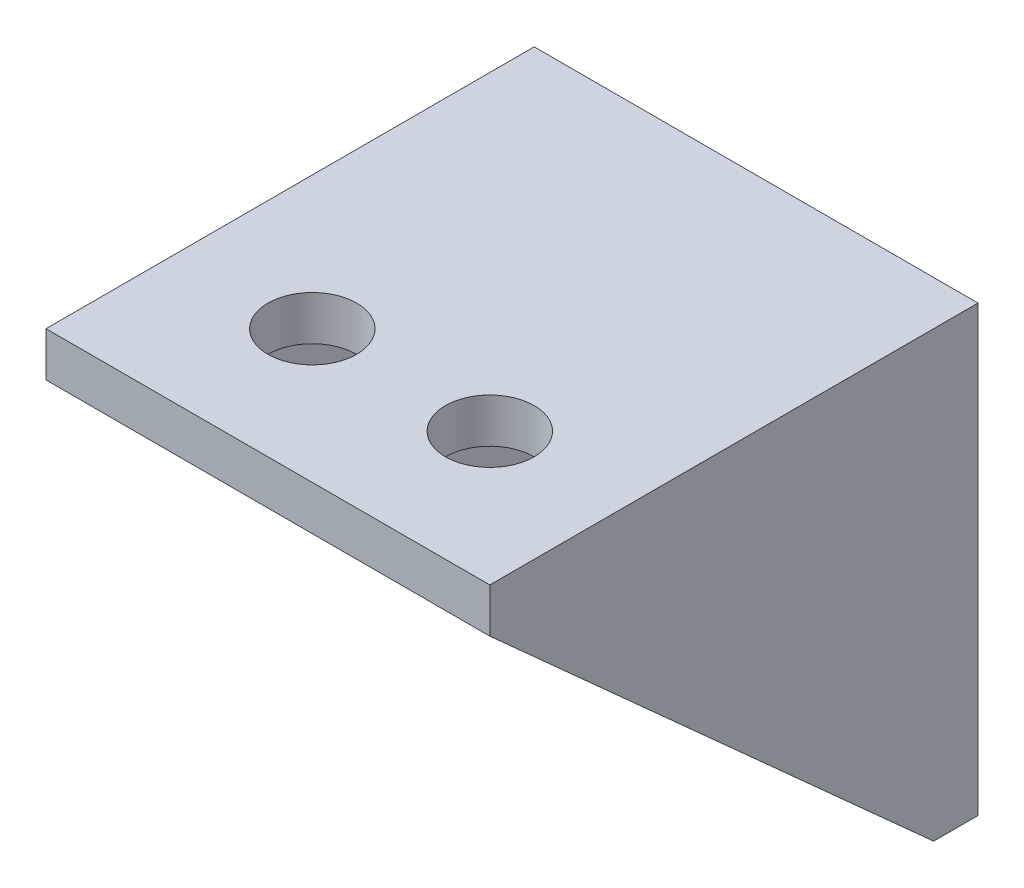
ISO-10303-21;
HEADER;
FILE_DESCRIPTION(('STEP AP214'),'2;1');
FILE_NAME('part.step','',(''),(''),'','','');
FILE_SCHEMA(('AUTOMOTIVE_DESIGN { 1 0 10303 214 1 1 1 1 }'));
ENDSEC;
DATA;
#1=APPLICATION_CONTEXT('core data for automotive mechanical design processes');
#2=APPLICATION_PROTOCOL_DEFINITION('international standard','automotive_design',2000,#1);
#3=PRODUCT_CONTEXT('',#1,'mechanical');
#4=PRODUCT('Part','Part','',(#3));
#5=PRODUCT_RELATED_PRODUCT_CATEGORY('part','',(#4));
#6=PRODUCT_DEFINITION_FORMATION('','',#4);
#7=PRODUCT_DEFINITION_CONTEXT('part definition',#1,'design');
#8=PRODUCT_DEFINITION('design','',#6,#7);
#9=PRODUCT_DEFINITION_SHAPE('','',#8);
#10=(LENGTH_UNIT() NAMED_UNIT(*) SI_UNIT(.MILLI.,.METRE.));
#11=(NAMED_UNIT(*) PLANE_ANGLE_UNIT() SI_UNIT($,.RADIAN.));
#12=(NAMED_UNIT(*) SI_UNIT($,.STERADIAN.) SOLID_ANGLE_UNIT());
#13=UNCERTAINTY_MEASURE_WITH_UNIT(LENGTH_MEASURE(1.E-05),#10,'distance_accuracy_value','');
#14=(GEOMETRIC_REPRESENTATION_CONTEXT(3) GLOBAL_UNCERTAINTY_ASSIGNED_CONTEXT((#13)) GLOBAL_UNIT_ASSIGNED_CONTEXT((#10,
#11,#12)) REPRESENTATION_CONTEXT('',''));
#15=CARTESIAN_POINT('',(0.,0.,0.));
#16=DIRECTION('',(0.,0.,1.));
#17=DIRECTION('',(1.,0.,0.));
#18=AXIS2_PLACEMENT_3D('',#15,#16,#17);
#19=CARTESIAN_POINT('',(0.,0.,12.7));
#20=DIRECTION('',(0.,0.,-1.));
#21=DIRECTION('',(-1.,0.,0.));
#22=AXIS2_PLACEMENT_3D('',#19,#20,#21);
#23=PLANE('',#22);
#24=CARTESIAN_POINT('',(91.0635678000014,25.4,12.7));
#25=DIRECTION('',(0.,0.,1.));
#26=DIRECTION('',(1.,0.,0.));
#27=AXIS2_PLACEMENT_3D('',#24,#25,#26);
#28=CIRCLE('',#27,12.7);
#29=CARTESIAN_POINT('',(103.763567800001,25.4,12.7));
#30=VERTEX_POINT('',#29);
#31=EDGE_CURVE('E430',#30,#30,#28,.T.);
#32=ORIENTED_EDGE('',*,*,#31,.F.);
#33=EDGE_LOOP('',(#32));
#34=FACE_BOUND('',#33,.T.);
#35=CARTESIAN_POINT('',(37.7740033866654,25.4,12.7));
#36=DIRECTION('',(0.,0.,1.));
#37=DIRECTION('',(1.,0.,0.));
#38=AXIS2_PLACEMENT_3D('',#35,#36,#37);
#39=CIRCLE('',#38,12.7);
#40=CARTESIAN_POINT('',(50.4740033866654,25.4,12.7));
#41=VERTEX_POINT('',#40);
#42=EDGE_CURVE('E427',#41,#41,#39,.T.);
#43=ORIENTED_EDGE('',*,*,#42,.F.);
#44=EDGE_LOOP('',(#43));
#45=FACE_BOUND('',#44,.T.);
#46=DIRECTION('',(0.,1.,0.));
#47=VECTOR('',#46,1.);
#48=CARTESIAN_POINT('',(114.3,0.,12.7));
#49=LINE('',#48,#47);
#50=CARTESIAN_POINT('',(114.3,0.,12.7));
#51=VERTEX_POINT('',#50);
#52=CARTESIAN_POINT('',(114.3,114.3,12.7));
#53=VERTEX_POINT('',#52);
#54=EDGE_CURVE('E114',#51,#53,#49,.T.);
#55=ORIENTED_EDGE('',*,*,#54,.T.);
#56=DIRECTION('',(1.,0.,0.));
#57=VECTOR('',#56,1.);
#58=CARTESIAN_POINT('',(0.,114.3,12.7));
#59=LINE('',#58,#57);
#60=CARTESIAN_POINT('',(12.7,114.3,12.7));
#61=VERTEX_POINT('',#60);
#62=EDGE_CURVE('E149',#61,#53,#59,.T.);
#63=ORIENTED_EDGE('',*,*,#62,.F.);
#64=DIRECTION('',(0.,-1.,0.));
#65=VECTOR('',#64,1.);
#66=CARTESIAN_POINT('',(12.7,114.3,12.7));
#67=LINE('',#66,#65);
#68=CARTESIAN_POINT('',(12.7,0.,12.7));
#69=VERTEX_POINT('',#68);
#70=EDGE_CURVE('E143',#61,#69,#67,.T.);
#71=ORIENTED_EDGE('',*,*,#70,.T.);
#72=DIRECTION('',(1.,0.,0.));
#73=VECTOR('',#72,1.);
#74=CARTESIAN_POINT('',(127.,0.,12.7));
#75=LINE('',#74,#73);
#76=EDGE_CURVE('E138',#69,#51,#75,.T.);
#77=ORIENTED_EDGE('',*,*,#76,.T.);
#78=EDGE_LOOP('',(#55,#63,#71,#77));
#79=FACE_BOUND('',#78,.T.);
#80=ADVANCED_FACE('F44',(#34,#45,#79),#23,.F.);
#81=CARTESIAN_POINT('',(0.,114.3,139.7));
#82=DIRECTION('',(0.,1.,0.));
#83=DIRECTION('',(0.,0.,1.));
#84=AXIS2_PLACEMENT_3D('',#81,#82,#83);
#85=PLANE('',#84);
#86=CARTESIAN_POINT('',(88.9,114.3,101.6));
#87=DIRECTION('',(0.,-1.,0.));
#88=DIRECTION('',(0.,0.,-1.));
#89=AXIS2_PLACEMENT_3D('',#86,#87,#88);
#90=CIRCLE('',#89,12.7);
#91=CARTESIAN_POINT('',(88.9,114.3,88.9));
#92=VERTEX_POINT('',#91);
#93=EDGE_CURVE('E434',#92,#92,#90,.T.);
#94=ORIENTED_EDGE('',*,*,#93,.F.);
#95=EDGE_LOOP('',(#94));
#96=FACE_BOUND('',#95,.T.);
#97=CARTESIAN_POINT('',(38.1,114.3,101.6));
#98=DIRECTION('',(0.,-1.,0.));
#99=DIRECTION('',(0.,0.,-1.));
#100=AXIS2_PLACEMENT_3D('',#97,#98,#99);
#101=CIRCLE('',#100,12.7);
#102=CARTESIAN_POINT('',(38.1,114.3,88.9));
#103=VERTEX_POINT('',#102);
#104=EDGE_CURVE('E194',#103,#103,#101,.T.);
#105=ORIENTED_EDGE('',*,*,#104,.F.);
#106=EDGE_LOOP('',(#105));
#107=FACE_BOUND('',#106,.T.);
#108=DIRECTION('',(0.,0.,1.));
#109=VECTOR('',#108,1.);
#110=CARTESIAN_POINT('',(114.3,114.3,12.7));
#111=LINE('',#110,#109);
#112=CARTESIAN_POINT('',(114.3,114.3,139.7));
#113=VERTEX_POINT('',#112);
#114=EDGE_CURVE('E118',#53,#113,#111,.T.);
#115=ORIENTED_EDGE('',*,*,#114,.T.);
#116=DIRECTION('',(1.,0.,0.));
#117=VECTOR('',#116,1.);
#118=CARTESIAN_POINT('',(0.,114.3,139.7));
#119=LINE('',#118,#117);
#120=CARTESIAN_POINT('',(12.7,114.3,139.7));
#121=VERTEX_POINT('',#120);
#122=EDGE_CURVE('E184',#121,#113,#119,.T.);
#123=ORIENTED_EDGE('',*,*,#122,.F.);
#124=DIRECTION('',(0.,0.,-1.));
#125=VECTOR('',#124,1.);
#126=CARTESIAN_POINT('',(12.7,114.3,139.7));
#127=LINE('',#126,#125);
#128=EDGE_CURVE('E58',#121,#61,#127,.T.);
#129=ORIENTED_EDGE('',*,*,#128,.T.);
#130=ORIENTED_EDGE('',*,*,#62,.T.);
#131=EDGE_LOOP('',(#115,#123,#129,#130));
#132=FACE_BOUND('',#131,.T.);
#133=ADVANCED_FACE('F201',(#96,#107,#132),#85,.F.);
#134=CARTESIAN_POINT('',(127.,0.,12.7));
#135=DIRECTION('',(0.,1.,0.));
#136=DIRECTION('',(0.,0.,1.));
#137=AXIS2_PLACEMENT_3D('',#134,#135,#136);
#138=PLANE('',#137);
#139=DIRECTION('',(1.,0.,0.));
#140=VECTOR('',#139,1.);
#141=CARTESIAN_POINT('',(127.,0.,0.));
#142=LINE('',#141,#140);
#143=CARTESIAN_POINT('',(0.,0.,0.));
#144=VERTEX_POINT('',#143);
#145=CARTESIAN_POINT('',(127.,0.,0.));
#146=VERTEX_POINT('',#145);
#147=EDGE_CURVE('E151',#144,#146,#142,.T.);
#148=ORIENTED_EDGE('',*,*,#147,.T.);
#149=DIRECTION('',(0.,0.,-1.));
#150=VECTOR('',#149,1.);
#151=CARTESIAN_POINT('',(127.,0.,12.7));
#152=LINE('',#151,#150);
#153=CARTESIAN_POINT('',(127.,0.,12.7));
#154=VERTEX_POINT('',#153);
#155=EDGE_CURVE('E11',#154,#146,#152,.T.);
#156=ORIENTED_EDGE('',*,*,#155,.F.);
#157=DIRECTION('',(1.,0.,0.));
#158=VECTOR('',#157,1.);
#159=CARTESIAN_POINT('',(114.3,0.,12.7));
#160=LINE('',#159,#158);
#161=EDGE_CURVE('E130',#51,#154,#160,.T.);
#162=ORIENTED_EDGE('',*,*,#161,.F.);
#163=ORIENTED_EDGE('',*,*,#76,.F.);
#164=CARTESIAN_POINT('',(0.,0.,12.7));
#165=VERTEX_POINT('',#164);
#166=EDGE_CURVE('E142',#165,#69,#75,.T.);
#167=ORIENTED_EDGE('',*,*,#166,.F.);
#168=DIRECTION('',(0.,0.,-1.));
#169=VECTOR('',#168,1.);
#170=CARTESIAN_POINT('',(0.,0.,12.7));
#171=LINE('',#170,#169);
#172=EDGE_CURVE('E145',#165,#144,#171,.T.);
#173=ORIENTED_EDGE('',*,*,#172,.T.);
#174=EDGE_LOOP('',(#148,#156,#162,#163,#167,#173));
#175=FACE_BOUND('',#174,.T.);
#176=ADVANCED_FACE('F50',(#175),#138,.F.);
#177=CARTESIAN_POINT('',(127.,127.,12.7));
#178=DIRECTION('',(-1.,0.,0.));
#179=DIRECTION('',(0.,0.,1.));
#180=AXIS2_PLACEMENT_3D('',#177,#178,#179);
#181=PLANE('',#180);
#182=DIRECTION('',(0.,1.,0.));
#183=VECTOR('',#182,1.);
#184=CARTESIAN_POINT('',(127.,127.,0.));
#185=LINE('',#184,#183);
#186=CARTESIAN_POINT('',(127.,127.,0.));
#187=VERTEX_POINT('',#186);
#188=EDGE_CURVE('E153',#146,#187,#185,.T.);
#189=ORIENTED_EDGE('',*,*,#188,.T.);
#190=DIRECTION('',(0.,0.,-1.));
#191=VECTOR('',#190,1.);
#192=CARTESIAN_POINT('',(127.,127.,12.7));
#193=LINE('',#192,#191);
#194=CARTESIAN_POINT('',(127.,127.,139.7));
#195=VERTEX_POINT('',#194);
#196=EDGE_CURVE('E52',#195,#187,#193,.T.);
#197=ORIENTED_EDGE('',*,*,#196,.F.);
#198=DIRECTION('',(0.,1.,0.));
#199=VECTOR('',#198,1.);
#200=CARTESIAN_POINT('',(127.,127.,139.7));
#201=LINE('',#200,#199);
#202=CARTESIAN_POINT('',(127.,114.3,139.7));
#203=VERTEX_POINT('',#202);
#204=EDGE_CURVE('E189',#203,#195,#201,.T.);
#205=ORIENTED_EDGE('',*,*,#204,.F.);
#206=DIRECTION('',(0.,-0.66896473162245,-0.743294146247166));
#207=VECTOR('',#206,1.);
#208=CARTESIAN_POINT('',(127.,114.3,139.7));
#209=LINE('',#208,#207);
#210=EDGE_CURVE('E132',#203,#154,#209,.T.);
#211=ORIENTED_EDGE('',*,*,#210,.T.);
#212=ORIENTED_EDGE('',*,*,#155,.T.);
#213=EDGE_LOOP('',(#189,#197,#205,#211,#212));
#214=FACE_BOUND('',#213,.T.);
#215=ADVANCED_FACE('F186',(#214),#181,.F.);
#216=CARTESIAN_POINT('',(0.,127.,12.7));
#217=DIRECTION('',(0.,-1.,0.));
#218=DIRECTION('',(0.,0.,-1.));
#219=AXIS2_PLACEMENT_3D('',#216,#217,#218);
#220=PLANE('',#219);
#221=CARTESIAN_POINT('',(88.9,127.,101.6));
#222=DIRECTION('',(0.,-1.,0.));
#223=DIRECTION('',(0.,0.,-1.));
#224=AXIS2_PLACEMENT_3D('',#221,#222,#223);
#225=CIRCLE('',#224,12.7);
#226=CARTESIAN_POINT('',(88.9,127.,88.9));
#227=VERTEX_POINT('',#226);
#228=EDGE_CURVE('E437',#227,#227,#225,.T.);
#229=ORIENTED_EDGE('',*,*,#228,.T.);
#230=EDGE_LOOP('',(#229));
#231=FACE_BOUND('',#230,.T.);
#232=CARTESIAN_POINT('',(38.1,127.,101.6));
#233=DIRECTION('',(0.,-1.,0.));
#234=DIRECTION('',(0.,0.,-1.));
#235=AXIS2_PLACEMENT_3D('',#232,#233,#234);
#236=CIRCLE('',#235,12.7);
#237=CARTESIAN_POINT('',(38.1,127.,88.9));
#238=VERTEX_POINT('',#237);
#239=EDGE_CURVE('E192',#238,#238,#236,.T.);
#240=ORIENTED_EDGE('',*,*,#239,.T.);
#241=EDGE_LOOP('',(#240));
#242=FACE_BOUND('',#241,.T.);
#243=DIRECTION('',(-1.,0.,0.));
#244=VECTOR('',#243,1.);
#245=CARTESIAN_POINT('',(0.,127.,0.));
#246=LINE('',#245,#244);
#247=CARTESIAN_POINT('',(0.,127.,0.));
#248=VERTEX_POINT('',#247);
#249=EDGE_CURVE('E144',#187,#248,#246,.T.);
#250=ORIENTED_EDGE('',*,*,#249,.T.);
#251=DIRECTION('',(0.,0.,-1.));
#252=VECTOR('',#251,1.);
#253=CARTESIAN_POINT('',(0.,127.,12.7));
#254=LINE('',#253,#252);
#255=CARTESIAN_POINT('',(0.,127.,139.7));
#256=VERTEX_POINT('',#255);
#257=EDGE_CURVE('E158',#256,#248,#254,.T.);
#258=ORIENTED_EDGE('',*,*,#257,.F.);
#259=DIRECTION('',(-1.,0.,0.));
#260=VECTOR('',#259,1.);
#261=CARTESIAN_POINT('',(0.,127.,139.7));
#262=LINE('',#261,#260);
#263=EDGE_CURVE('E152',#195,#256,#262,.T.);
#264=ORIENTED_EDGE('',*,*,#263,.F.);
#265=ORIENTED_EDGE('',*,*,#196,.T.);
#266=EDGE_LOOP('',(#250,#258,#264,#265));
#267=FACE_BOUND('',#266,.T.);
#268=ADVANCED_FACE('F162',(#231,#242,#267),#220,.F.);
#269=CARTESIAN_POINT('',(0.,0.,12.7));
#270=DIRECTION('',(1.,0.,0.));
#271=DIRECTION('',(0.,0.,-1.));
#272=AXIS2_PLACEMENT_3D('',#269,#270,#271);
#273=PLANE('',#272);
#274=ORIENTED_EDGE('',*,*,#172,.F.);
#275=DIRECTION('',(0.,0.66896473162245,0.743294146247166));
#276=VECTOR('',#275,1.);
#277=CARTESIAN_POINT('',(0.,0.,12.7));
#278=LINE('',#277,#276);
#279=CARTESIAN_POINT('',(0.,114.3,139.7));
#280=VERTEX_POINT('',#279);
#281=EDGE_CURVE('E174',#165,#280,#278,.T.);
#282=ORIENTED_EDGE('',*,*,#281,.T.);
#283=DIRECTION('',(0.,-1.,0.));
#284=VECTOR('',#283,1.);
#285=CARTESIAN_POINT('',(0.,127.,139.7));
#286=LINE('',#285,#284);
#287=EDGE_CURVE('E177',#256,#280,#286,.T.);
#288=ORIENTED_EDGE('',*,*,#287,.F.);
#289=ORIENTED_EDGE('',*,*,#257,.T.);
#290=DIRECTION('',(0.,-1.,0.));
#291=VECTOR('',#290,1.);
#292=CARTESIAN_POINT('',(0.,0.,0.));
#293=LINE('',#292,#291);
#294=EDGE_CURVE('E68',#248,#144,#293,.T.);
#295=ORIENTED_EDGE('',*,*,#294,.T.);
#296=EDGE_LOOP('',(#274,#282,#288,#289,#295));
#297=FACE_BOUND('',#296,.T.);
#298=ADVANCED_FACE('F175',(#297),#273,.F.);
#299=CARTESIAN_POINT('',(0.,0.,0.));
#300=DIRECTION('',(0.,0.,-1.));
#301=DIRECTION('',(-1.,0.,0.));
#302=AXIS2_PLACEMENT_3D('',#299,#300,#301);
#303=PLANE('',#302);
#304=CARTESIAN_POINT('',(91.0635678000014,25.4,0.));
#305=DIRECTION('',(0.,0.,1.));
#306=DIRECTION('',(1.,0.,0.));
#307=AXIS2_PLACEMENT_3D('',#304,#305,#306);
#308=CIRCLE('',#307,12.7);
#309=CARTESIAN_POINT('',(103.763567800001,25.4,0.));
#310=VERTEX_POINT('',#309);
#311=EDGE_CURVE('E424',#310,#310,#308,.T.);
#312=ORIENTED_EDGE('',*,*,#311,.T.);
#313=EDGE_LOOP('',(#312));
#314=FACE_BOUND('',#313,.T.);
#315=CARTESIAN_POINT('',(37.7740033866654,25.4,0.));
#316=DIRECTION('',(0.,0.,1.));
#317=DIRECTION('',(1.,0.,0.));
#318=AXIS2_PLACEMENT_3D('',#315,#316,#317);
#319=CIRCLE('',#318,12.7);
#320=CARTESIAN_POINT('',(50.4740033866654,25.4,0.));
#321=VERTEX_POINT('',#320);
#322=EDGE_CURVE('E435',#321,#321,#319,.T.);
#323=ORIENTED_EDGE('',*,*,#322,.T.);
#324=EDGE_LOOP('',(#323));
#325=FACE_BOUND('',#324,.T.);
#326=ORIENTED_EDGE('',*,*,#147,.F.);
#327=ORIENTED_EDGE('',*,*,#294,.F.);
#328=ORIENTED_EDGE('',*,*,#249,.F.);
#329=ORIENTED_EDGE('',*,*,#188,.F.);
#330=EDGE_LOOP('',(#326,#327,#328,#329));
#331=FACE_BOUND('',#330,.T.);
#332=ADVANCED_FACE('F168',(#314,#325,#331),#303,.T.);
#333=CARTESIAN_POINT('',(0.,0.,139.7));
#334=DIRECTION('',(0.,0.,1.));
#335=DIRECTION('',(1.,0.,0.));
#336=AXIS2_PLACEMENT_3D('',#333,#334,#335);
#337=PLANE('',#336);
#338=ORIENTED_EDGE('',*,*,#287,.T.);
#339=EDGE_CURVE('E181',#280,#121,#119,.T.);
#340=ORIENTED_EDGE('',*,*,#339,.T.);
#341=ORIENTED_EDGE('',*,*,#122,.T.);
#342=DIRECTION('',(1.,0.,0.));
#343=VECTOR('',#342,1.);
#344=CARTESIAN_POINT('',(114.3,114.3,139.7));
#345=LINE('',#344,#343);
#346=EDGE_CURVE('E128',#113,#203,#345,.T.);
#347=ORIENTED_EDGE('',*,*,#346,.T.);
#348=ORIENTED_EDGE('',*,*,#204,.T.);
#349=ORIENTED_EDGE('',*,*,#263,.T.);
#350=EDGE_LOOP('',(#338,#340,#341,#347,#348,#349));
#351=FACE_BOUND('',#350,.T.);
#352=ADVANCED_FACE('F182',(#351),#337,.T.);
#353=CARTESIAN_POINT('',(12.7,0.,12.7));
#354=DIRECTION('',(0.,-0.743294146247166,0.66896473162245));
#355=DIRECTION('',(0.,-0.66896473162245,-0.743294146247166));
#356=AXIS2_PLACEMENT_3D('',#353,#354,#355);
#357=PLANE('',#356);
#358=ORIENTED_EDGE('',*,*,#281,.F.);
#359=ORIENTED_EDGE('',*,*,#166,.T.);
#360=DIRECTION('',(0.,0.66896473162245,0.743294146247166));
#361=VECTOR('',#360,1.);
#362=CARTESIAN_POINT('',(12.7,0.,12.7));
#363=LINE('',#362,#361);
#364=EDGE_CURVE('E199',#69,#121,#363,.T.);
#365=ORIENTED_EDGE('',*,*,#364,.T.);
#366=ORIENTED_EDGE('',*,*,#339,.F.);
#367=EDGE_LOOP('',(#358,#359,#365,#366));
#368=FACE_BOUND('',#367,.T.);
#369=ADVANCED_FACE('F240',(#368),#357,.T.);
#370=CARTESIAN_POINT('',(12.7,0.,0.));
#371=DIRECTION('',(1.,0.,0.));
#372=DIRECTION('',(0.,0.,-1.));
#373=AXIS2_PLACEMENT_3D('',#370,#371,#372);
#374=PLANE('',#373);
#375=ORIENTED_EDGE('',*,*,#70,.F.);
#376=ORIENTED_EDGE('',*,*,#128,.F.);
#377=ORIENTED_EDGE('',*,*,#364,.F.);
#378=EDGE_LOOP('',(#375,#376,#377));
#379=FACE_BOUND('',#378,.T.);
#380=ADVANCED_FACE('F238',(#379),#374,.T.);
#381=CARTESIAN_POINT('',(114.3,114.3,139.7));
#382=DIRECTION('',(0.,-0.743294146247166,0.66896473162245));
#383=DIRECTION('',(0.,-0.66896473162245,-0.743294146247166));
#384=AXIS2_PLACEMENT_3D('',#381,#382,#383);
#385=PLANE('',#384);
#386=ORIENTED_EDGE('',*,*,#210,.F.);
#387=ORIENTED_EDGE('',*,*,#346,.F.);
#388=DIRECTION('',(0.,-0.66896473162245,-0.743294146247166));
#389=VECTOR('',#388,1.);
#390=CARTESIAN_POINT('',(114.3,114.3,139.7));
#391=LINE('',#390,#389);
#392=EDGE_CURVE('E117',#113,#51,#391,.T.);
#393=ORIENTED_EDGE('',*,*,#392,.T.);
#394=ORIENTED_EDGE('',*,*,#161,.T.);
#395=EDGE_LOOP('',(#386,#387,#393,#394));
#396=FACE_BOUND('',#395,.T.);
#397=ADVANCED_FACE('F127',(#396),#385,.T.);
#398=CARTESIAN_POINT('',(114.3,0.,0.));
#399=DIRECTION('',(1.,0.,0.));
#400=DIRECTION('',(0.,0.,-1.));
#401=AXIS2_PLACEMENT_3D('',#398,#399,#400);
#402=PLANE('',#401);
#403=ORIENTED_EDGE('',*,*,#392,.F.);
#404=ORIENTED_EDGE('',*,*,#114,.F.);
#405=ORIENTED_EDGE('',*,*,#54,.F.);
#406=EDGE_LOOP('',(#403,#404,#405));
#407=FACE_BOUND('',#406,.T.);
#408=ADVANCED_FACE('F113',(#407),#402,.F.);
#409=CARTESIAN_POINT('',(38.1,127.,101.6));
#410=DIRECTION('',(0.,-1.,0.));
#411=DIRECTION('',(0.,0.,-1.));
#412=AXIS2_PLACEMENT_3D('',#409,#410,#411);
#413=CYLINDRICAL_SURFACE('',#412,12.7);
#414=ORIENTED_EDGE('',*,*,#239,.F.);
#415=EDGE_LOOP('',(#414));
#416=FACE_BOUND('',#415,.T.);
#417=ORIENTED_EDGE('',*,*,#104,.T.);
#418=EDGE_LOOP('',(#417));
#419=FACE_BOUND('',#418,.T.);
#420=ADVANCED_FACE('F256',(#416,#419),#413,.F.);
#421=CARTESIAN_POINT('',(88.9,127.,101.6));
#422=DIRECTION('',(0.,-1.,0.));
#423=DIRECTION('',(0.,0.,-1.));
#424=AXIS2_PLACEMENT_3D('',#421,#422,#423);
#425=CYLINDRICAL_SURFACE('',#424,12.7);
#426=ORIENTED_EDGE('',*,*,#228,.F.);
#427=EDGE_LOOP('',(#426));
#428=FACE_BOUND('',#427,.T.);
#429=ORIENTED_EDGE('',*,*,#93,.T.);
#430=EDGE_LOOP('',(#429));
#431=FACE_BOUND('',#430,.T.);
#432=ADVANCED_FACE('F264',(#428,#431),#425,.F.);
#433=CARTESIAN_POINT('',(37.7740033866654,25.4,0.));
#434=DIRECTION('',(0.,0.,1.));
#435=DIRECTION('',(1.,0.,0.));
#436=AXIS2_PLACEMENT_3D('',#433,#434,#435);
#437=CYLINDRICAL_SURFACE('',#436,12.7);
#438=ORIENTED_EDGE('',*,*,#322,.F.);
#439=EDGE_LOOP('',(#438));
#440=FACE_BOUND('',#439,.T.);
#441=ORIENTED_EDGE('',*,*,#42,.T.);
#442=EDGE_LOOP('',(#441));
#443=FACE_BOUND('',#442,.T.);
#444=ADVANCED_FACE('F275',(#440,#443),#437,.F.);
#445=CARTESIAN_POINT('',(91.0635678000014,25.4,0.));
#446=DIRECTION('',(0.,0.,1.));
#447=DIRECTION('',(1.,0.,0.));
#448=AXIS2_PLACEMENT_3D('',#445,#446,#447);
#449=CYLINDRICAL_SURFACE('',#448,12.7);
#450=ORIENTED_EDGE('',*,*,#311,.F.);
#451=EDGE_LOOP('',(#450));
#452=FACE_BOUND('',#451,.T.);
#453=ORIENTED_EDGE('',*,*,#31,.T.);
#454=EDGE_LOOP('',(#453));
#455=FACE_BOUND('',#454,.T.);
#456=ADVANCED_FACE('F278',(#452,#455),#449,.F.);
#457=CLOSED_SHELL('',(#80,#133,#176,#215,#268,#298,#332,#352,#369,#380,#397,#408,#420,#432,#444,#456));
#458=MANIFOLD_SOLID_BREP('B2',#457);
#459=ADVANCED_BREP_SHAPE_REPRESENTATION('',(#18,#458),#14);
#460=SHAPE_DEFINITION_REPRESENTATION(#9,#459);
ENDSEC;
END-ISO-10303-21;
